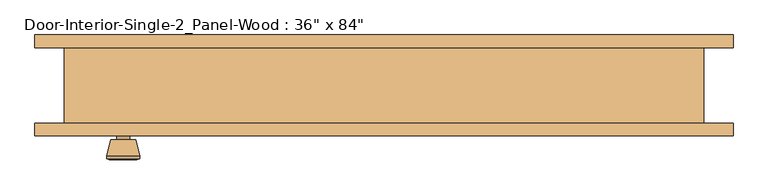
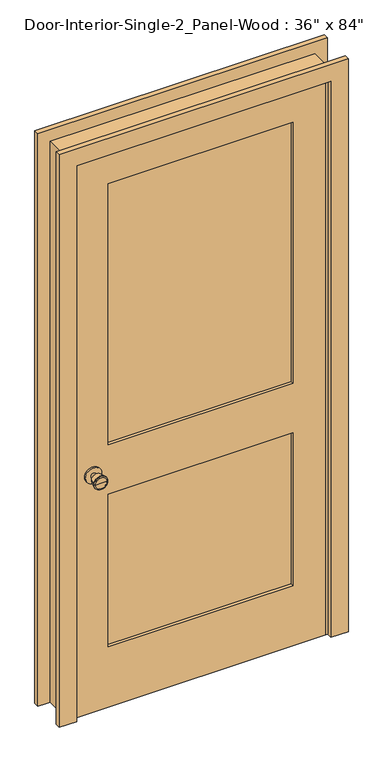
"""IFC4 building model written with IfcOpenShell, lengths in millimetres: door geometry."""

from ifc_helpers import new_model, si_unit, point, frame, frame_2d, origin, place, context, project, spatial, polyline, circle_curve, trimmed, segment, composite_curve, outline, extrude, faceted_brep, source, transform, mapped, element, save
from ifc_brep_helpers import plane_surface, cylinder_surface, revolved_surface, advanced_brep


def door_049a69ed(model_context):
    return source(origin(), model_context, "Body", "SolidModel", [
        advanced_brep(
        [(-393.7, -13.05, 914.4), (-403.7, -13.05, 914.4), (-383.7, -13.05, 914.4), (-373.2241324, 35.95, 914.4), (-414.1758676, 35.95, 914.4), (-393.7, 35.95, 914.4), (-368.7, 34.1221319, 914.4), (-418.7, 34.1221319, 914.4), (-368.7, 30.6584537, 914.4), (-418.7, 30.6584537, 914.4), (-375.063764, 5.95, 914.4), (-412.336236, 5.95, 914.4), (-383.7, 5.95, 914.4), (-403.7, 5.95, 914.4)],
        [
            (0, 1),
            (1, 2, circle_curve(frame((-393.7, -13.05, 914.4), z_axis=(0.0, -1.0, 0.0), x_axis=(-1.0, 0.0, 0.0)), 10.0)),
            (2, 0),
            (2, 1, circle_curve(frame((-393.7, -13.05, 914.4), z_axis=(0.0, -1.0, 0.0), x_axis=(-1.0, 0.0, 0.0)), 10.0)),
            (3, 4, circle_curve(frame((-393.7, 35.95, 914.4), z_axis=(0.0, 1.0, 0.0), x_axis=(-1.0, 0.0, 0.0)), 20.4758676)),
            (4, 5),
            (5, 3),
            (4, 3, circle_curve(frame((-393.7, 35.95, 914.4), z_axis=(0.0, 1.0, 0.0), x_axis=(-1.0, 0.0, 0.0)), 20.4758676)),
            (6, 7, circle_curve(frame((-393.7, 34.1221319, 914.4), z_axis=(0.0, 1.0, 0.0), x_axis=(-1.0, 0.0, 0.0)), 25.0)),
            (7, 4),
            (3, 6),
            (7, 6, circle_curve(frame((-393.7, 34.1221319, 914.4), z_axis=(0.0, 1.0, 0.0), x_axis=(-1.0, 0.0, 0.0)), 25.0)),
            (8, 9, circle_curve(frame((-393.7, 30.6584537, 914.4), z_axis=(0.0, 1.0, 0.0), x_axis=(-1.0, 0.0, 0.0)), 25.0)),
            (9, 7),
            (6, 8),
            (9, 8, circle_curve(frame((-393.7, 30.6584537, 914.4), z_axis=(0.0, 1.0, 0.0), x_axis=(-1.0, 0.0, 0.0)), 25.0)),
            (10, 11, circle_curve(frame((-393.7, 5.95, 914.4), z_axis=(0.0, 1.0, 0.0), x_axis=(-1.0, 0.0, 0.0)), 18.636236)),
            (11, 9),
            (8, 10),
            (11, 10, circle_curve(frame((-393.7, 5.95, 914.4), z_axis=(0.0, 1.0, 0.0), x_axis=(-1.0, 0.0, 0.0)), 18.636236)),
            (12, 13, circle_curve(frame((-393.7, 5.95, 914.4), z_axis=(0.0, 1.0, 0.0), x_axis=(-1.0, 0.0, 0.0)), 10.0)),
            (13, 11),
            (10, 12),
            (13, 12, circle_curve(frame((-393.7, 5.95, 914.4), z_axis=(0.0, 1.0, 0.0), x_axis=(-1.0, 0.0, 0.0)), 10.0)),
            (1, 13),
            (12, 2),
        ],
        [
            plane_surface(frame((-393.7, -13.05, 914.4), z_axis=(0.0, -1.0, 0.0), x_axis=(-1.0, 0.0, 0.0))),
            plane_surface(frame((-393.7, 35.95, 914.4), z_axis=(0.0, 1.0, 0.0), x_axis=(-1.0, 0.0, 0.0))),
            revolved_surface(polyline([(-414.1758676, 35.95, 914.4), (-418.7, 34.1221319, 914.4)]), (-393.7, -13.05, 914.4), (0.0, -1.0, 0.0)),
            cylinder_surface(frame((-393.7, -13.05, 914.4), z_axis=(0.0, -1.0, 0.0), x_axis=(-1.0, 0.0, 0.0)), 25.0),
            revolved_surface(polyline([(-418.7, 30.6584537, 914.4), (-412.336236, 5.95, 914.4)]), (-393.7, -13.05, 914.4), (0.0, -1.0, 0.0)),
            plane_surface(frame((-393.7, 5.95, 914.4), z_axis=(0.0, -1.0, 0.0), x_axis=(-1.0, 0.0, 0.0))),
            cylinder_surface(frame((-393.7, -13.05, 914.4), z_axis=(0.0, -1.0, 0.0), x_axis=(-1.0, 0.0, 0.0)), 10.0),
        ],
        [
            (0, [[1, 2, 3]]),
            (0, [[-3, 4, -1]]),
            (1, [[5, 6, 7]]),
            (1, [[8, -7, -6]]),
            (2, [[9, 10, -5, 11]]),
            (2, [[12, -11, -8, -10]]),
            (3, [[13, 14, -9, 15]]),
            (3, [[16, -15, -12, -14]]),
            (4, [[17, 18, -13, 19]]),
            (4, [[20, -19, -16, -18]]),
            (5, [[21, 22, -17, 23]]),
            (5, [[24, -23, -20, -22]]),
            (6, [[-2, 25, -21, 26]]),
            (6, [[-4, -26, -24, -25]]),
        ],
    ),
        extrude(outline(composite_curve([segment(trimmed(circle_curve(frame_2d((914.4, -393.7)), 30.0), [point((914.4, -423.7))], [point((914.4, -363.7))], False, "CARTESIAN"), True, "CONTINUOUS"), segment(trimmed(circle_curve(frame_2d((914.4, -393.7)), 30.0), [point((914.4, -363.7))], [point((914.4, -423.7))], False, "CARTESIAN"), True, "CONTINUOUS")], self_intersect=False)), frame((0.0, -19.05, 0.0), z_axis=(0.0, 1.0, 0.0), x_axis=(0.0, 0.0, 1.0)), (0.0, 0.0, 1.0), 6.0),
        advanced_brep(
        [(-393.7, -59.975, 914.4), (-383.7, -59.975, 914.4), (-403.7, -59.975, 914.4), (-373.2241324, -108.975, 914.4), (-393.7, -108.975, 914.4), (-414.1758676, -108.975, 914.4), (-368.7, -107.1471319, 914.4), (-418.7, -107.1471319, 914.4), (-368.7, -103.6834537, 914.4), (-418.7, -103.6834537, 914.4), (-375.063764, -78.975, 914.4), (-412.336236, -78.975, 914.4), (-383.7, -78.975, 914.4), (-403.7, -78.975, 914.4)],
        [
            (0, 1),
            (1, 2, circle_curve(frame((-393.7, -59.975, 914.4), z_axis=(0.0, 1.0, 0.0), x_axis=(-1.0, 0.0, 0.0)), 10.0)),
            (2, 0),
            (2, 1, circle_curve(frame((-393.7, -59.975, 914.4), z_axis=(0.0, 1.0, 0.0), x_axis=(-1.0, 0.0, 0.0)), 10.0)),
            (3, 4),
            (4, 5),
            (5, 3, circle_curve(frame((-393.7, -108.975, 914.4), z_axis=(0.0, -1.0, 0.0), x_axis=(-1.0, 0.0, 0.0)), 20.4758676)),
            (3, 5, circle_curve(frame((-393.7, -108.975, 914.4), z_axis=(0.0, -1.0, 0.0), x_axis=(-1.0, 0.0, 0.0)), 20.4758676)),
            (6, 3),
            (5, 7),
            (7, 6, circle_curve(frame((-393.7, -107.1471319, 914.4), z_axis=(0.0, -1.0, 0.0), x_axis=(-1.0, 0.0, 0.0)), 25.0)),
            (6, 7, circle_curve(frame((-393.7, -107.1471319, 914.4), z_axis=(0.0, -1.0, 0.0), x_axis=(-1.0, 0.0, 0.0)), 25.0)),
            (8, 6),
            (7, 9),
            (9, 8, circle_curve(frame((-393.7, -103.6834537, 914.4), z_axis=(0.0, -1.0, 0.0), x_axis=(-1.0, 0.0, 0.0)), 25.0)),
            (8, 9, circle_curve(frame((-393.7, -103.6834537, 914.4), z_axis=(0.0, -1.0, 0.0), x_axis=(-1.0, 0.0, 0.0)), 25.0)),
            (10, 8),
            (9, 11),
            (11, 10, circle_curve(frame((-393.7, -78.975, 914.4), z_axis=(0.0, -1.0, 0.0), x_axis=(-1.0, 0.0, 0.0)), 18.636236)),
            (10, 11, circle_curve(frame((-393.7, -78.975, 914.4), z_axis=(0.0, -1.0, 0.0), x_axis=(-1.0, 0.0, 0.0)), 18.636236)),
            (12, 10),
            (11, 13),
            (13, 12, circle_curve(frame((-393.7, -78.975, 914.4), z_axis=(0.0, -1.0, 0.0), x_axis=(-1.0, 0.0, 0.0)), 10.0)),
            (12, 13, circle_curve(frame((-393.7, -78.975, 914.4), z_axis=(0.0, -1.0, 0.0), x_axis=(-1.0, 0.0, 0.0)), 10.0)),
            (1, 12),
            (13, 2),
        ],
        [
            plane_surface(frame((-393.7, -59.975, 914.4), z_axis=(0.0, 1.0, 0.0), x_axis=(-1.0, 0.0, 0.0))),
            plane_surface(frame((-393.7, -108.975, 914.4), z_axis=(0.0, -1.0, 0.0), x_axis=(-1.0, 0.0, 0.0))),
            revolved_surface(polyline([(-414.1758676, -108.975, 914.4), (-418.7, -107.1471319, 914.4)]), (-393.7, -59.975, 914.4), (0.0, 1.0, 0.0)),
            cylinder_surface(frame((-393.7, -59.975, 914.4), z_axis=(0.0, 1.0, 0.0), x_axis=(-1.0, 0.0, 0.0)), 25.0),
            revolved_surface(polyline([(-418.7, -103.6834537, 914.4), (-412.336236, -78.975, 914.4)]), (-393.7, -59.975, 914.4), (0.0, 1.0, 0.0)),
            plane_surface(frame((-393.7, -78.975, 914.4), z_axis=(0.0, 1.0, 0.0), x_axis=(-1.0, 0.0, 0.0))),
            cylinder_surface(frame((-393.7, -59.975, 914.4), z_axis=(0.0, 1.0, 0.0), x_axis=(-1.0, 0.0, 0.0)), 10.0),
        ],
        [
            (0, [[1, 2, 3]]),
            (0, [[-3, 4, -1]]),
            (1, [[5, 6, 7]]),
            (1, [[-6, -5, 8]]),
            (2, [[9, -7, 10, 11]]),
            (2, [[-10, -8, -9, 12]]),
            (3, [[13, -11, 14, 15]]),
            (3, [[-14, -12, -13, 16]]),
            (4, [[17, -15, 18, 19]]),
            (4, [[-18, -16, -17, 20]]),
            (5, [[21, -19, 22, 23]]),
            (5, [[-22, -20, -21, 24]]),
            (6, [[25, -23, 26, -2]]),
            (6, [[-26, -24, -25, -4]]),
        ],
    ),
        extrude(outline(composite_curve([segment(trimmed(circle_curve(frame_2d((914.4, -393.7)), 30.0), [point((914.4, -423.7))], [point((914.4, -363.7))], False, "CARTESIAN"), True, "CONTINUOUS"), segment(trimmed(circle_curve(frame_2d((914.4, -393.7)), 30.0), [point((914.4, -363.7))], [point((914.4, -423.7))], False, "CARTESIAN"), True, "CONTINUOUS")], self_intersect=False)), frame((0.0, -59.975, 0.0), z_axis=(0.0, 1.0, 0.0), x_axis=(0.0, 0.0, 1.0)), (0.0, 0.0, 1.0), 6.0),
        faceted_brep([(482.6, -53.975, 0.0), (457.2, -53.975, 0.0), (457.2, -19.05, 0.0), (444.5, -19.05, 0.0), (444.5, 15.875, 0.0), (457.2, 15.875, 0.0), (457.2, 60.325, 0.0), (482.6, 60.325, 0.0), (482.6, 60.325, 2159.0), (482.6, -53.975, 2159.0), (457.2, 60.325, 2133.6), (-457.2, 60.325, 2133.6), (-457.2, 60.325, 0.0), (-482.6, 60.325, 0.0), (-482.6, 60.325, 2159.0), (457.2, 15.875, 2133.6), (444.5, 15.875, 2120.9), (-444.5, 15.875, 2120.9), (-444.5, 15.875, 0.0), (-457.2, 15.875, 0.0), (-457.2, 15.875, 2133.6), (444.5, -19.05, 2120.9), (457.2, -19.05, 2133.6), (-457.2, -19.05, 2133.6), (-457.2, -19.05, 0.0), (-444.5, -19.05, 0.0), (-444.5, -19.05, 2120.9), (457.2, -53.975, 2133.6), (-482.6, -53.975, 2159.0), (-482.6, -53.975, 0.0), (-457.2, -53.975, 0.0), (-457.2, -53.975, 2133.6)], [[[0, 1, 2, 3, 4, 5, 6, 7]], [[7, 8, 9, 0]], [[6, 10, 11, 12, 13, 14, 8, 7]], [[5, 15, 10, 6]], [[4, 16, 17, 18, 19, 20, 15, 5]], [[3, 21, 16, 4]], [[2, 22, 23, 24, 25, 26, 21, 3]], [[1, 27, 22, 2]], [[0, 9, 28, 29, 30, 31, 27, 1]], [[8, 14, 28, 9]], [[15, 20, 11, 10]], [[21, 26, 17, 16]], [[27, 31, 23, 22]], [[29, 13, 12, 19, 18, 25, 24, 30]], [[14, 13, 29, 28]], [[20, 19, 12, 11]], [[26, 25, 18, 17]], [[31, 30, 24, 23]]]),
        extrude(outline(polyline([(2133.6, -457.2), (0.0, -457.2), (0.0, 457.2), (2133.6, 457.2), (2133.6, -457.2)]), holes=[polyline([(2014.5375, -336.55), (2014.5375, 336.55), (1009.65, 336.55), (1009.65, -336.55), (2014.5375, -336.55)]), polyline([(819.15, -336.55), (819.15, 336.55), (231.775, 336.55), (231.775, -336.55), (819.15, -336.55)])]), frame((0.0, -53.975, 0.0), z_axis=(0.0, 1.0, 0.0), x_axis=(0.0, 0.0, 1.0)), (0.0, 0.0, 1.0), 34.925),
        extrude(outline(polyline([(336.55, -30.6916667), (336.55, -42.3333333), (-336.55, -42.3333333), (-336.55, -30.6916667), (336.55, -30.6916667)])), frame((0.0, 0.0, 1009.65), z_axis=(0.0, 0.0, 1.0), x_axis=(1.0, 0.0, 0.0)), (0.0, 0.0, 1.0), 1004.8875),
        extrude(outline(polyline([(336.55, -30.6916667), (336.55, -42.3333333), (-336.55, -42.3333333), (-336.55, -30.6916667), (336.55, -30.6916667)])), frame((0.0, 0.0, 231.775), z_axis=(0.0, 0.0, 1.0), x_axis=(1.0, 0.0, 0.0)), (0.0, 0.0, 1.0), 587.375),
        extrude(outline(polyline([(0.0, 527.05), (2203.45, 527.05), (2203.45, -527.05), (0.0, -527.05), (0.0, -463.55), (2139.95, -463.55), (2139.95, 463.55), (0.0, 463.55), (0.0, 527.05)])), frame((0.0, -73.025, 0.0), z_axis=(0.0, 1.0, 0.0), x_axis=(0.0, 0.0, 1.0)), (0.0, 0.0, 1.0), 19.05),
        extrude(outline(polyline([(0.0, 527.05), (2203.45, 527.05), (2203.45, -527.05), (0.0, -527.05), (0.0, -463.55), (2139.95, -463.55), (2139.95, 463.55), (0.0, 463.55), (0.0, 527.05)])), frame((0.0, 60.325, 0.0), z_axis=(0.0, 1.0, 0.0), x_axis=(0.0, 0.0, 1.0)), (0.0, 0.0, 1.0), 19.05),
    ])


if __name__ == "__main__":
    model = new_model("IFC4")
    model_context = context("Model", 3, world=origin())
    ifc_project = project(units=[si_unit("LENGTHUNIT", "METRE", prefix="MILLI")], contexts=[model_context])
    site = spatial("IfcSite", under=ifc_project)
    building = spatial("IfcBuilding", under=site)
    placement = place(None, origin())
    door_shape = door_049a69ed(model_context)
    element("IfcDoor", 1, ObjectType="Door-Interior-Single-2_Panel-Wood : 36\" x 84\"", at=placement, inside=building, context=model_context, shape_type="MappedRepresentation", body=[
        mapped(door_shape, transform((0.0, 0.0, 0.0), x_axis=(1.0, 0.0, 0.0), y_axis=(0.0, 1.0, 0.0), z_axis=(0.0, 0.0, 1.0))),
    ])
    save(model, "model.ifc")

# Revit data of these elements
# Type "Door-Interior-Single-2_Panel-Wood : 36\" x 84\""
#   Type Mark = "12"
#   Assembly Code = "C1020300"
#   Analytic Construction = "Wooden"
#   Top Rail = 0' - 4 11/16"
#   Thickness = 0' - 1 3/8"
#   Thermal Resistance (R) = 2.5876 (h·ft²·°F)/BTU
#   Swing Angle [instance default] = 90.00°
#   Stiles = 0' - 4 3/4"
#   Rough Width = 3' - 2"
#   Rough Height = 7' - 1"
#   Lock Rail = 0' - 7 1/2"
#   Height = 7' - 0"
#   Width = 3' - 0"
#   Heat Transfer Coefficient (U) = 0.3865 BTU/(h·ft²·°F)
#   Bottom Rail = 0' - 9 1/8"
#   Trim Material = Cherry
#   Panel Material = Cherry
#   Frame Material = Cherry
#   Door Handle Material = Aluminum
#   Visual Light Transmittance = 0
#   Solar Heat Gain Coefficient = 0
#   Wall Closure = (empty or 0)
#   Function = (empty or 0)
# Element 1 (IfcDoor, "Door-Interior-Single-2_Panel-Wood : 36\" x 84\"")
#   Materials on its faces: "Cherry", "Aluminum"
# Materials
#   "Cherry": class "Wood", colour RGB 226 177 128, transparency 0, Description = "Prunus Serotina", Cost = 0
#   "Aluminum": class "Metal", colour RGB 247 247 247, transparency 0, Description = "Aluminum 6061", Cost = 0
